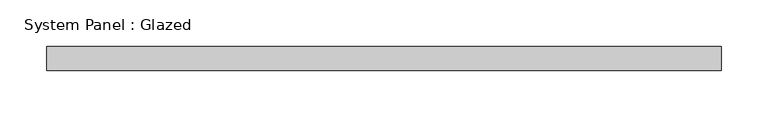
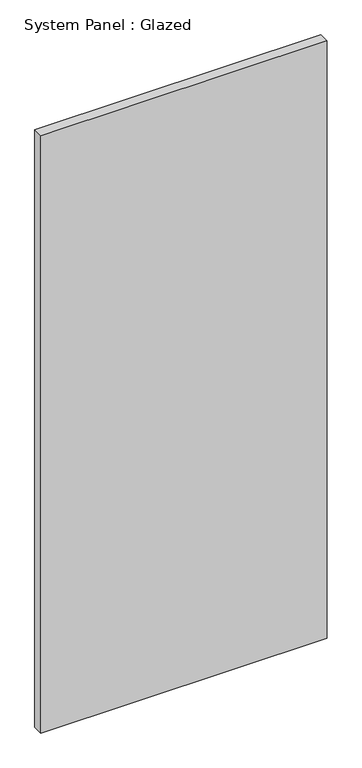
"""IFC4 building model written with IfcOpenShell, lengths in millimetres: plate geometry, System Panel : Glazed."""

from ifc_helpers import new_model, si_unit, origin, origin_with_axes, place, context, project, spatial, polyline, outline, extrude, source, transform, mapped, element, save


def system_panel_glazed_1cc22cd7(model_context):
    return source(origin(), model_context, "Body", "SweptSolid", [
        extrude(outline(polyline([(358.775, 19.05), (-358.775, 19.05), (-358.775, 44.45), (358.775, 44.45), (358.775, 19.05)])), origin_with_axes(), (0.0, 0.0, 1.0), 1581.8911809),
    ])


if __name__ == "__main__":
    model = new_model("IFC4")
    model_context = context("Model", 3, world=origin())
    ifc_project = project(units=[si_unit("LENGTHUNIT", "METRE", prefix="MILLI")], contexts=[model_context])
    site = spatial("IfcSite", under=ifc_project)
    building = spatial("IfcBuilding", under=site)
    placement = place(None, origin())
    system_panel_glazed_shape = system_panel_glazed_1cc22cd7(model_context)
    element("IfcPlate", 1, ObjectType="System Panel : Glazed", at=placement, inside=building, context=model_context, shape_type="MappedRepresentation", body=[
        mapped(system_panel_glazed_shape, transform((0.0, 0.0, 0.0), x_axis=(1.0, 0.0, 0.0), y_axis=(0.0, 1.0, 0.0), z_axis=(0.0, 0.0, 1.0))),
    ])
    save(model, "model.ifc")

# Revit data of these elements
# Type "System Panel : Glazed"
#   Construction Type Id = "GSP4R"
#   Analytic Construction = "1/8 in Pilkington single glazing"
#   Visual Light Transmittance = 0.9
#   Solar Heat Gain Coefficient = 0.86
#   Heat Transfer Coefficient (U) = 1.18115 BTU/(h·ft²·°F)
#   Define Thermal Properties by = 1
# Element 1 (IfcPlate, "System Panel : Glazed")
#   Materials on its faces: "Glass"
# Materials
#   "Glass": class "Glass", colour RGB 0 128 192, transparency 0.75, Description = "Soda Lime Glass", Cost = 0
